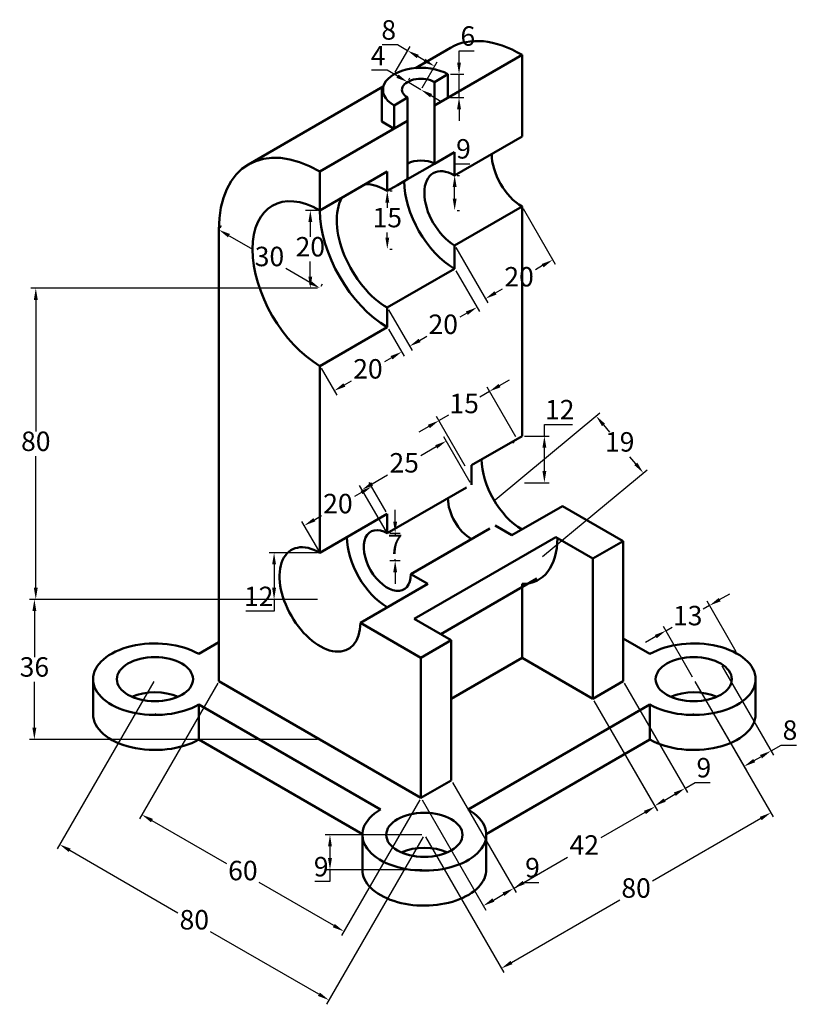
# Model space of a CAD drawing. Units: millimetres. Extents: x 11 to 211, y -6 to 247.
import ezdxf

# ---------------------------------------------------------------- set-up
doc = ezdxf.new("R2010")
doc.units = ezdxf.units.MM
doc.layers.add('M-DIMS', color=2, linetype='Continuous', lineweight=25)
doc.layers.add('M-OUTL', color=7, linetype='Continuous', lineweight=50)
doc.styles.get("Standard").update_dxf_attribs({"font": 'arial.ttf'})
doc.dimstyles.new('ISO-25', dxfattribs={"dimtxt": 5, "dimasz": 3, "dimexe": 1.25, "dimexo": 0.625, "dimtad": 1, "dimtih": 1, "dimtoh": 1, "dimtxsty": 'Standard', "dimcen": 2.5, "dimadec": 0, "dimazin": 0, "dimtfac": 1, "dimtmove": 0, "dimatfit": 3, "dimfxl": 1, "dimarcsym": 0})

# ---------------------------------------------------------------- blocks, each defined once
blk = doc.blocks.new('*D1')
at = {"layer": 'Defpoints', "color": 0, "transparency": 16777216}
for p in [(183.96, 77.16), (203.77, 42.84), (114.67, 37.16)]:
    blk.add_point(p, dxfattribs=at)
at = {"layer": 'M-DIMS', "color": 0, "lineweight": -2, "transparency": 16777216}
for p, q in [((184.27, 76.61), (204.39, 41.76)), ((201.17, 41.34), (173.33, 25.27)), ((114.99, 36.61), (135.11, 1.76)), ((137.08, 4.34), (164.93, 20.41))]:
    blk.add_line(p, q, dxfattribs=at)
at = {"layer": 'M-DIMS', "color": 0, "transparency": 16777216}
for points in [[(200.92, 41.77), (201.42, 40.91), (203.77, 42.84)], [(136.83, 4.77), (137.33, 3.91), (134.49, 2.84)]]:
    blk.add_solid(points, dxfattribs=at)
at = {"layer": 'M-DIMS', "color": 0, "transparency": 16777216, "insert": (169.13, 22.84), "char_height": 5, "attachment_point": 5}
blk.add_mtext('80', dxfattribs=at)
blk = doc.blocks.new('*D2')
at = {"layer": 'Defpoints', "color": 0, "transparency": 16777216}
for p in [(157.98, 72.16), (121.6, 51.16), (174, 44.4)]:
    blk.add_point(p, dxfattribs=at)
at = {"layer": 'M-DIMS', "color": 0, "lineweight": -2, "transparency": 16777216}
for p, q in [((158.29, 71.61), (174.62, 43.32)), ((121.91, 50.61), (138.25, 22.32)), ((171.4, 42.9), (160.09, 36.37)), ((140.22, 24.9), (151.53, 31.43))]:
    blk.add_line(p, q, dxfattribs=at)
at = {"layer": 'M-DIMS', "color": 0, "transparency": 16777216}
for points in [[(171.15, 43.33), (171.65, 42.47), (174, 44.4)], [(139.97, 25.33), (140.47, 24.47), (137.63, 23.4)]]:
    blk.add_solid(points, dxfattribs=at)
at = {"layer": 'M-DIMS', "color": 0, "transparency": 16777216, "insert": (155.81, 33.9), "char_height": 5, "attachment_point": 5}
blk.add_mtext('42', dxfattribs=at)
blk = doc.blocks.new('*D3')
at = {"layer": 'Defpoints', "color": 0, "transparency": 16777216}
for p in [(121.6, 51.16), (113.81, 46.66), (137.63, 23.4)]:
    blk.add_point(p, dxfattribs=at)
at = {"layer": 'M-DIMS', "color": 0, "lineweight": -2, "transparency": 16777216}
for p, q in [((121.91, 50.61), (138.25, 22.32)), ((114.12, 46.11), (130.46, 17.82)), ((137.63, 23.4), (140.22, 24.9)), ((140.22, 24.9), (144.14, 24.9)), ((132.43, 20.4), (135.03, 21.9))]:
    blk.add_line(p, q, dxfattribs=at)
at = {"layer": 'M-DIMS', "color": 0, "transparency": 16777216}
for points in [[(134.78, 22.33), (135.28, 21.47), (137.63, 23.4)], [(132.18, 20.83), (132.68, 19.97), (129.83, 18.9)]]:
    blk.add_solid(points, dxfattribs=at)
at = {"layer": 'M-DIMS', "color": 0, "transparency": 16777216, "insert": (142.49, 28.08), "char_height": 5, "attachment_point": 5}
blk.add_mtext('9', dxfattribs=at)
blk = doc.blocks.new('*D4')
at = {"layer": 'Defpoints', "color": 0, "transparency": 16777216}
for p in [(165.77, 76.66), (157.98, 72.16), (181.68, 49.09)]:
    blk.add_point(p, dxfattribs=at)
at = {"layer": 'M-DIMS', "color": 0, "lineweight": -2, "transparency": 16777216}
for p, q in [((166.08, 76.11), (182.31, 48.01)), ((158.29, 71.61), (174.51, 43.51)), ((181.68, 49.09), (184.28, 50.59)), ((184.28, 50.59), (188.19, 50.59)), ((176.49, 46.09), (179.08, 47.59))]:
    blk.add_line(p, q, dxfattribs=at)
at = {"layer": 'M-DIMS', "color": 0, "transparency": 16777216}
for points in [[(178.83, 48.03), (179.33, 47.16), (181.68, 49.09)], [(176.24, 46.53), (176.74, 45.66), (173.89, 44.59)]]:
    blk.add_solid(points, dxfattribs=at)
at = {"layer": 'M-DIMS', "color": 0, "transparency": 16777216, "insert": (186.55, 53.77), "char_height": 5, "attachment_point": 5}
blk.add_mtext('9', dxfattribs=at)
blk = doc.blocks.new('*D5')
at = {"layer": 'Defpoints', "color": 0, "transparency": 16777216}
for p in [(114.67, 37.16), (90.41, 28.16), (114.67, 28.16)]:
    blk.add_point(p, dxfattribs=at)
at = {"layer": 'M-DIMS', "color": 0, "lineweight": -2, "transparency": 16777216}
for p, q in [((114.05, 37.16), (89.16, 37.16)), ((90.41, 34.16), (90.41, 31.16)), ((114.05, 28.16), (89.16, 28.16)), ((90.41, 28.16), (90.41, 25.16)), ((90.41, 25.16), (86.49, 25.16))]:
    blk.add_line(p, q, dxfattribs=at)
at = {"layer": 'M-DIMS', "color": 0, "transparency": 16777216}
for points in [[(89.91, 34.16), (90.91, 34.16), (90.41, 37.16)], [(89.91, 31.16), (90.91, 31.16), (90.41, 28.16)]]:
    blk.add_solid(points, dxfattribs=at)
at = {"layer": 'M-DIMS', "color": 0, "transparency": 16777216, "insert": (88.14, 28.33), "char_height": 5, "attachment_point": 5}
blk.add_mtext('9', dxfattribs=at)
blk = doc.blocks.new('*D6')
at = {"layer": 'Defpoints', "color": 0, "transparency": 16777216}
for p in [(45.39, 77.16), (114.67, 37.16), (90.15, -5.32)]:
    blk.add_point(p, dxfattribs=at)
at = {"layer": 'M-DIMS', "color": 0, "lineweight": -2, "transparency": 16777216}
for p, q in [((45.08, 76.61), (20.24, 33.6)), ((114.36, 36.61), (89.53, -6.4)), ((23.47, 33.18), (51.31, 17.1)), ((87.55, -3.82), (59.71, 12.25))]:
    blk.add_line(p, q, dxfattribs=at)
at = {"layer": 'M-DIMS', "color": 0, "transparency": 16777216}
for points in [[(23.72, 33.61), (23.22, 32.75), (20.87, 34.68)], [(87.8, -3.39), (87.3, -4.25), (90.15, -5.32)]]:
    blk.add_solid(points, dxfattribs=at)
at = {"layer": 'M-DIMS', "color": 0, "transparency": 16777216, "insert": (55.51, 14.68), "char_height": 5, "attachment_point": 5}
blk.add_mtext('80', dxfattribs=at)
blk = doc.blocks.new('*D7')
at = {"layer": 'Defpoints', "color": 0, "transparency": 16777216}
for p in [(61.85, 76.66), (113.81, 46.66), (93.99, 12.33)]:
    blk.add_point(p, dxfattribs=at)
at = {"layer": 'M-DIMS', "color": 0, "lineweight": -2, "transparency": 16777216}
for p, q in [((61.53, 76.11), (41.4, 41.24)), ((113.5, 46.11), (93.36, 11.24)), ((44.62, 40.83), (63.8, 29.76)), ((91.39, 13.83), (72.22, 24.89))]:
    blk.add_line(p, q, dxfattribs=at)
at = {"layer": 'M-DIMS', "color": 0, "transparency": 16777216}
for points in [[(44.87, 41.26), (44.37, 40.39), (42.03, 42.33)], [(91.64, 14.26), (91.14, 13.39), (93.99, 12.33)]]:
    blk.add_solid(points, dxfattribs=at)
at = {"layer": 'M-DIMS', "color": 0, "transparency": 16777216, "insert": (68.01, 27.33), "char_height": 5, "attachment_point": 5}
blk.add_mtext('60', dxfattribs=at)
blk = doc.blocks.new('*D8')
at = {"layer": 'Defpoints', "color": 0, "transparency": 16777216}
for p in [(87.83, 177.66), (14.75, 97.66), (87.83, 97.66)]:
    blk.add_point(p, dxfattribs=at)
at = {"layer": 'M-DIMS', "color": 0, "lineweight": -2, "transparency": 16777216}
for p, q in [((87.2, 177.66), (13.5, 177.66)), ((14.75, 174.66), (14.75, 140.83)), ((14.75, 100.66), (14.75, 134.48)), ((87.2, 97.66), (13.5, 97.66))]:
    blk.add_line(p, q, dxfattribs=at)
at = {"layer": 'M-DIMS', "color": 0, "transparency": 16777216}
for points in [[(14.25, 174.66), (15.25, 174.66), (14.75, 177.66)], [(14.25, 100.66), (15.25, 100.66), (14.75, 97.66)]]:
    blk.add_solid(points, dxfattribs=at)
at = {"layer": 'M-DIMS', "color": 0, "transparency": 16777216, "insert": (14.75, 137.66), "char_height": 5, "attachment_point": 5}
blk.add_mtext('80', dxfattribs=at)
blk = doc.blocks.new('*D9')
at = {"layer": 'Defpoints', "color": 0, "transparency": 16777216}
for p in [(87.83, 97.66), (14.39, 61.66), (87.83, 61.66)]:
    blk.add_point(p, dxfattribs=at)
at = {"layer": 'M-DIMS', "color": 0, "lineweight": -2, "transparency": 16777216}
for p, q in [((87.2, 97.66), (13.14, 97.66)), ((14.39, 94.66), (14.39, 82.84)), ((14.39, 64.66), (14.39, 76.48)), ((87.2, 61.66), (13.14, 61.66))]:
    blk.add_line(p, q, dxfattribs=at)
at = {"layer": 'M-DIMS', "color": 0, "transparency": 16777216}
for points in [[(13.89, 94.66), (14.89, 94.66), (14.39, 97.66)], [(13.89, 64.66), (14.89, 64.66), (14.39, 61.66)]]:
    blk.add_solid(points, dxfattribs=at)
at = {"layer": 'M-DIMS', "color": 0, "transparency": 16777216, "insert": (14.39, 79.66), "char_height": 5, "attachment_point": 5}
blk.add_mtext('36', dxfattribs=at)
blk = doc.blocks.new('*D10')
at = {"layer": 'Defpoints', "color": 0, "transparency": 16777216}
for p in [(87.83, 109.66), (76.03, 97.66), (87.83, 97.66)]:
    blk.add_point(p, dxfattribs=at)
at = {"layer": 'M-DIMS', "color": 0, "lineweight": -2, "transparency": 16777216}
for p, q in [((87.2, 109.66), (74.78, 109.66)), ((76.03, 106.66), (76.03, 100.66)), ((87.2, 97.66), (74.78, 97.66)), ((76.03, 97.66), (76.03, 94.66)), ((76.03, 94.66), (68.76, 94.66))]:
    blk.add_line(p, q, dxfattribs=at)
at = {"layer": 'M-DIMS', "color": 0, "transparency": 16777216}
for points in [[(75.53, 106.66), (76.53, 106.66), (76.03, 109.66)], [(75.53, 100.66), (76.53, 100.66), (76.03, 97.66)]]:
    blk.add_solid(points, dxfattribs=at)
at = {"layer": 'M-DIMS', "color": 0, "transparency": 16777216, "insert": (72.08, 97.79), "char_height": 5, "attachment_point": 5}
blk.add_mtext('12', dxfattribs=at)
blk = doc.blocks.new('*D11')
at = {"layer": 'Defpoints', "color": 0, "transparency": 16777216}
for p in [(105.15, 114.66), (107.17, 114.66), (105.15, 107.66)]:
    blk.add_point(p, dxfattribs=at)
at = {"layer": 'M-DIMS', "color": 0, "lineweight": -2, "transparency": 16777216}
for p, q in [((107.17, 117.66), (107.17, 120.66)), ((105.77, 114.66), (108.42, 114.66)), ((107.17, 114.66), (107.17, 114.28)), ((105.77, 107.66), (108.42, 107.66)), ((107.17, 107.66), (107.17, 108.03)), ((107.17, 104.66), (107.17, 101.66))]:
    blk.add_line(p, q, dxfattribs=at)
at = {"layer": 'M-DIMS', "color": 0, "transparency": 16777216}
for points in [[(106.67, 117.66), (107.67, 117.66), (107.17, 114.66)], [(106.67, 104.66), (107.67, 104.66), (107.17, 107.66)]]:
    blk.add_solid(points, dxfattribs=at)
at = {"layer": 'M-DIMS', "color": 0, "transparency": 16777216, "insert": (107.17, 111.16), "char_height": 5, "attachment_point": 5}
blk.add_mtext('7', dxfattribs=at)
blk = doc.blocks.new('*D12')
at = {"layer": 'Defpoints', "color": 0, "transparency": 16777216}
for p in [(101.11, 126.65), (105.15, 119.66), (87.83, 109.66)]:
    blk.add_point(p, dxfattribs=at)
at = {"layer": 'M-DIMS', "color": 0, "lineweight": -2, "transparency": 16777216}
for p, q in [((104.84, 120.2), (100.49, 127.73)), ((98.51, 125.15), (96.69, 124.1)), ((86.39, 118.15), (88.21, 119.2)), ((87.51, 110.2), (83.16, 117.73))]:
    blk.add_line(p, q, dxfattribs=at)
at = {"layer": 'M-DIMS', "color": 0, "transparency": 16777216}
for points in [[(98.26, 125.58), (98.76, 124.72), (101.11, 126.65)], [(86.14, 118.58), (86.64, 117.72), (83.79, 116.65)]]:
    blk.add_solid(points, dxfattribs=at)
at = {"layer": 'M-DIMS', "color": 0, "transparency": 16777216, "insert": (92.45, 121.65), "char_height": 5, "attachment_point": 5}
blk.add_mtext('20', dxfattribs=at)
blk = doc.blocks.new('*D13')
at = {"layer": 'Defpoints', "color": 0, "transparency": 16777216}
for p in [(120.32, 138.38), (126.8, 127.16), (105.15, 114.66)]:
    blk.add_point(p, dxfattribs=at)
at = {"layer": 'M-DIMS', "color": 0, "lineweight": -2, "transparency": 16777216}
for p, q in [((126.49, 127.7), (119.69, 139.46)), ((117.72, 136.88), (113.76, 134.59)), ((101.27, 127.38), (105.23, 129.67)), ((104.84, 115.2), (98.04, 126.96))]:
    blk.add_line(p, q, dxfattribs=at)
at = {"layer": 'M-DIMS', "color": 0, "transparency": 16777216}
for points in [[(117.47, 137.31), (117.97, 136.45), (120.32, 138.38)], [(101.02, 127.81), (101.52, 126.95), (98.67, 125.88)]]:
    blk.add_solid(points, dxfattribs=at)
at = {"layer": 'M-DIMS', "color": 0, "transparency": 16777216, "insert": (109.49, 132.13), "char_height": 5, "attachment_point": 5}
blk.add_mtext('25', dxfattribs=at)
blk = doc.blocks.new('*D14')
at = {"layer": 'Defpoints', "color": 0, "transparency": 16777216}
for p in [(131.42, 151.13), (138.48, 138.9), (125.49, 131.4)]:
    blk.add_point(p, dxfattribs=at)
at = {"layer": 'M-DIMS', "color": 0, "lineweight": -2, "transparency": 16777216}
for p, q in [((138.16, 139.44), (130.79, 152.21)), ((134.02, 152.63), (136.61, 154.13)), ((131.42, 151.13), (128.91, 149.68)), ((125.17, 131.94), (117.8, 144.71)), ((118.43, 143.63), (120.93, 145.07)), ((115.83, 142.13), (113.23, 140.63))]:
    blk.add_line(p, q, dxfattribs=at)
at = {"layer": 'M-DIMS', "color": 0, "transparency": 16777216}
for points in [[(133.77, 153.06), (134.27, 152.19), (131.42, 151.13)], [(115.58, 142.56), (116.08, 141.69), (118.43, 143.63)]]:
    blk.add_solid(points, dxfattribs=at)
at = {"layer": 'M-DIMS', "color": 0, "transparency": 16777216, "insert": (124.92, 147.38), "char_height": 5, "attachment_point": 5}
blk.add_mtext('15', dxfattribs=at)
blk = doc.blocks.new('*D15')
at = {"layer": 'Defpoints', "color": 0, "transparency": 16777216}
for p in [(139.79, 139.66), (145.55, 139.66), (139.79, 127.66)]:
    blk.add_point(p, dxfattribs=at)
at = {"layer": 'M-DIMS', "color": 0, "lineweight": -2, "transparency": 16777216}
for p, q in [((145.55, 139.66), (145.55, 142.66)), ((145.55, 142.66), (152.81, 142.66)), ((140.41, 139.66), (146.8, 139.66)), ((145.55, 130.66), (145.55, 136.66)), ((140.41, 127.66), (146.8, 127.66))]:
    blk.add_line(p, q, dxfattribs=at)
at = {"layer": 'M-DIMS', "color": 0, "transparency": 16777216}
for points in [[(145.05, 136.66), (146.05, 136.66), (145.55, 139.66)], [(145.05, 130.66), (146.05, 130.66), (145.55, 127.66)]]:
    blk.add_solid(points, dxfattribs=at)
at = {"layer": 'M-DIMS', "color": 0, "transparency": 16777216, "insert": (149.49, 145.79), "char_height": 5, "attachment_point": 5}
blk.add_mtext('12', dxfattribs=at)
blk = doc.blocks.new('*D16')
at = {"layer": 'Defpoints', "color": 0, "transparency": 16777216}
for p in [(105.15, 167.66), (108.83, 161.28), (87.83, 157.66)]:
    blk.add_point(p, dxfattribs=at)
at = {"layer": 'M-DIMS', "color": 0, "lineweight": -2, "transparency": 16777216}
for p, q in [((105.46, 167.11), (109.45, 160.2)), ((106.23, 159.78), (104.41, 158.73)), ((88.14, 157.11), (92.13, 150.2)), ((94.1, 152.78), (95.93, 153.84))]:
    blk.add_line(p, q, dxfattribs=at)
at = {"layer": 'M-DIMS', "color": 0, "transparency": 16777216}
for points in [[(105.98, 160.22), (106.48, 159.35), (108.83, 161.28)], [(93.85, 153.22), (94.35, 152.35), (91.51, 151.28)]]:
    blk.add_solid(points, dxfattribs=at)
at = {"layer": 'M-DIMS', "color": 0, "transparency": 16777216, "insert": (100.17, 156.28), "char_height": 5, "attachment_point": 5}
blk.add_mtext('20', dxfattribs=at)
blk = doc.blocks.new('*D17')
at = {"layer": 'Defpoints', "color": 0, "transparency": 16777216}
for p in [(122.47, 182.66), (105.15, 172.66), (128.2, 172.74)]:
    blk.add_point(p, dxfattribs=at)
at = {"layer": 'M-DIMS', "color": 0, "lineweight": -2, "transparency": 16777216}
for p, q in [((122.78, 182.11), (128.82, 171.65)), ((105.46, 172.11), (111.5, 161.65)), ((125.6, 171.24), (123.78, 170.18)), ((113.47, 164.24), (115.29, 165.29))]:
    blk.add_line(p, q, dxfattribs=at)
at = {"layer": 'M-DIMS', "color": 0, "transparency": 16777216}
for points in [[(125.35, 171.67), (125.85, 170.8), (128.2, 172.74)], [(113.22, 164.67), (113.72, 163.8), (110.87, 162.74)]]:
    blk.add_solid(points, dxfattribs=at)
at = {"layer": 'M-DIMS', "color": 0, "transparency": 16777216, "insert": (119.53, 167.74), "char_height": 5, "attachment_point": 5}
blk.add_mtext('20', dxfattribs=at)
blk = doc.blocks.new('*D18')
at = {"layer": 'Defpoints', "color": 0, "transparency": 16777216}
for p in [(139.79, 198.66), (122.47, 188.66), (147.7, 184.95)]:
    blk.add_point(p, dxfattribs=at)
at = {"layer": 'M-DIMS', "color": 0, "lineweight": -2, "transparency": 16777216}
for p, q in [((140.1, 198.11), (148.33, 183.87)), ((122.78, 188.11), (131.01, 173.87)), ((145.1, 183.45), (143.28, 182.4)), ((132.98, 176.45), (134.8, 177.5))]:
    blk.add_line(p, q, dxfattribs=at)
at = {"layer": 'M-DIMS', "color": 0, "transparency": 16777216}
for points in [[(144.85, 183.88), (145.35, 183.02), (147.7, 184.95)], [(132.73, 176.88), (133.23, 176.02), (130.38, 174.95)]]:
    blk.add_solid(points, dxfattribs=at)
at = {"layer": 'M-DIMS', "color": 0, "transparency": 16777216, "insert": (139.04, 179.95), "char_height": 5, "attachment_point": 5}
blk.add_mtext('20', dxfattribs=at)
blk = doc.blocks.new('*D19')
at = {"layer": 'Defpoints', "color": 0, "transparency": 16777216}
for p in [(170.97, 130.2), (132.43, 122.9), (144.57, 108.28)]:
    blk.add_point(p, dxfattribs=at)
at = {"layer": 'M-DIMS', "color": 0, "lineweight": -2, "transparency": 16777216}
for p, q in [((132.92, 123.3), (159.8, 145.62)), ((160.76, 142.51), (162.27, 140.69)), ((169.06, 132.51), (167.54, 134.33)), ((145.05, 108.68), (171.94, 131))]:
    blk.add_line(p, q, dxfattribs=at)
at = {"layer": 'M-DIMS', "color": 0, "transparency": 16777216}
for points in [[(161.14, 142.83), (160.37, 142.19), (158.84, 144.82)], [(169.44, 132.83), (168.67, 132.19), (170.97, 130.2)]]:
    blk.add_solid(points, dxfattribs=at)
at = {"layer": 'M-DIMS', "color": 0, "transparency": 16777216, "insert": (164.91, 137.51), "char_height": 5, "attachment_point": 5}
blk.add_mtext('19', dxfattribs=at)
blk = doc.blocks.new('*D20')
at = {"layer": 'Defpoints', "color": 0, "transparency": 16777216}
for p in [(61.85, 192.66), (61.85, 192.66), (87.83, 177.66)]:
    blk.add_point(p, dxfattribs=at)
at = {"layer": 'M-DIMS', "color": 0, "lineweight": -2, "transparency": 16777216}
for p, q in [((62.16, 193.2), (62.47, 193.74)), ((64.44, 191.16), (70.64, 187.58)), ((85.23, 179.16), (79.03, 182.73)), ((88.14, 178.2), (88.45, 178.74))]:
    blk.add_line(p, q, dxfattribs=at)
at = {"layer": 'M-DIMS', "color": 0, "transparency": 16777216}
for points in [[(64.69, 191.59), (64.19, 190.72), (61.85, 192.66)], [(85.48, 179.59), (84.98, 178.72), (87.83, 177.66)]]:
    blk.add_solid(points, dxfattribs=at)
at = {"layer": 'M-DIMS', "color": 0, "transparency": 16777216, "insert": (74.84, 185.16), "char_height": 5, "attachment_point": 5}
blk.add_mtext('30', dxfattribs=at)
blk = doc.blocks.new('*D21')
at = {"layer": 'Defpoints', "color": 0, "transparency": 16777216}
for p in [(85.35, 197.66), (87.83, 197.66), (87.83, 177.66)]:
    blk.add_point(p, dxfattribs=at)
at = {"layer": 'M-DIMS', "color": 0, "lineweight": -2, "transparency": 16777216}
for p, q in [((87.2, 197.66), (84.1, 197.66)), ((85.35, 194.66), (85.35, 190.83)), ((85.35, 180.66), (85.35, 184.48)), ((87.2, 177.66), (84.1, 177.66))]:
    blk.add_line(p, q, dxfattribs=at)
at = {"layer": 'M-DIMS', "color": 0, "transparency": 16777216}
for points in [[(84.85, 194.66), (85.85, 194.66), (85.35, 197.66)], [(84.85, 180.66), (85.85, 180.66), (85.35, 177.66)]]:
    blk.add_solid(points, dxfattribs=at)
at = {"layer": 'M-DIMS', "color": 0, "transparency": 16777216, "insert": (85.35, 187.66), "char_height": 5, "attachment_point": 5}
blk.add_mtext('20', dxfattribs=at)
blk = doc.blocks.new('*D22')
at = {"layer": 'Defpoints', "color": 0, "transparency": 16777216}
for p in [(105.15, 202.66), (105.15, 202.66), (105.15, 187.66)]:
    blk.add_point(p, dxfattribs=at)
at = {"layer": 'M-DIMS', "color": 0, "lineweight": -2, "transparency": 16777216}
for p, q in [((105.77, 202.66), (106.4, 202.66)), ((105.15, 199.66), (105.15, 198.33)), ((105.15, 190.66), (105.15, 191.98)), ((105.77, 187.66), (106.4, 187.66))]:
    blk.add_line(p, q, dxfattribs=at)
at = {"layer": 'M-DIMS', "color": 0, "transparency": 16777216}
for points in [[(104.65, 199.66), (105.65, 199.66), (105.15, 202.66)], [(104.65, 190.66), (105.65, 190.66), (105.15, 187.66)]]:
    blk.add_solid(points, dxfattribs=at)
at = {"layer": 'M-DIMS', "color": 0, "transparency": 16777216, "insert": (105.15, 195.16), "char_height": 5, "attachment_point": 5}
blk.add_mtext('15', dxfattribs=at)
blk = doc.blocks.new('*D23')
at = {"layer": 'Defpoints', "color": 0, "transparency": 16777216}
for p in [(122.47, 206.66), (122.47, 206.66), (122.47, 197.66)]:
    blk.add_point(p, dxfattribs=at)
at = {"layer": 'M-DIMS', "color": 0, "lineweight": -2, "transparency": 16777216}
for p, q in [((122.47, 206.66), (122.47, 209.66)), ((122.47, 209.66), (126.38, 209.66)), ((123.09, 206.66), (123.72, 206.66)), ((122.47, 200.66), (122.47, 203.66)), ((123.09, 197.66), (123.72, 197.66))]:
    blk.add_line(p, q, dxfattribs=at)
at = {"layer": 'M-DIMS', "color": 0, "transparency": 16777216}
for points in [[(121.97, 203.66), (122.97, 203.66), (122.47, 206.66)], [(121.97, 200.66), (122.97, 200.66), (122.47, 197.66)]]:
    blk.add_solid(points, dxfattribs=at)
at = {"layer": 'M-DIMS', "color": 0, "transparency": 16777216, "insert": (124.74, 212.83), "char_height": 5, "attachment_point": 5}
blk.add_mtext('9', dxfattribs=at)
blk = doc.blocks.new('*D24')
at = {"layer": 'Defpoints', "color": 0, "transparency": 16777216}
for p in [(120.74, 232.66), (123.59, 232.66), (120.74, 226.66)]:
    blk.add_point(p, dxfattribs=at)
at = {"layer": 'M-DIMS', "color": 0, "lineweight": -2, "transparency": 16777216}
for p, q in [((123.59, 235.66), (123.59, 238.66)), ((123.59, 238.66), (127.51, 238.66)), ((121.36, 232.66), (124.84, 232.66)), ((123.59, 226.66), (123.59, 232.66)), ((121.36, 226.66), (124.84, 226.66)), ((123.59, 223.66), (123.59, 220.66))]:
    blk.add_line(p, q, dxfattribs=at)
at = {"layer": 'M-DIMS', "color": 0, "transparency": 16777216}
for points in [[(123.09, 235.66), (124.09, 235.66), (123.59, 232.66)], [(123.09, 223.66), (124.09, 223.66), (123.59, 226.66)]]:
    blk.add_solid(points, dxfattribs=at)
at = {"layer": 'M-DIMS', "color": 0, "transparency": 16777216, "insert": (125.86, 241.83), "char_height": 5, "attachment_point": 5}
blk.add_mtext('6', dxfattribs=at)
blk = doc.blocks.new('*D25')
at = {"layer": 'Defpoints', "color": 0, "transparency": 16777216}
for p in [(110.34, 230.66), (110.34, 230.66), (113.81, 228.66)]:
    blk.add_point(p, dxfattribs=at)
at = {"layer": 'M-DIMS', "color": 0, "lineweight": -2, "transparency": 16777216}
for p, q in [((105.15, 233.66), (101.06, 233.66)), ((107.75, 232.16), (105.15, 233.66)), ((113.81, 228.66), (110.34, 230.66)), ((110.66, 231.2), (110.97, 231.74)), ((114.12, 229.2), (114.43, 229.74)), ((116.41, 227.16), (119, 225.66))]:
    blk.add_line(p, q, dxfattribs=at)
at = {"layer": 'M-DIMS', "color": 0, "transparency": 16777216}
for points in [[(108, 232.59), (107.5, 231.72), (110.34, 230.66)], [(116.66, 227.59), (116.16, 226.72), (113.81, 228.66)]]:
    blk.add_solid(points, dxfattribs=at)
at = {"layer": 'M-DIMS', "color": 0, "transparency": 16777216, "insert": (102.79, 236.78), "char_height": 5, "attachment_point": 5}
blk.add_mtext('4', dxfattribs=at)
blk = doc.blocks.new('*D26')
at = {"layer": 'Defpoints', "color": 0, "transparency": 16777216}
for p in [(110.38, 238.71), (106.88, 232.66), (113.81, 228.66)]:
    blk.add_point(p, dxfattribs=at)
at = {"layer": 'M-DIMS', "color": 0, "lineweight": -2, "transparency": 16777216}
for p, q in [((107.78, 240.21), (103.86, 240.21)), ((107.19, 233.2), (111, 239.8)), ((110.38, 238.71), (107.78, 240.21)), ((114.71, 236.21), (112.98, 237.21)), ((114.12, 229.2), (117.93, 235.8))]:
    blk.add_line(p, q, dxfattribs=at)
at = {"layer": 'M-DIMS', "color": 0, "transparency": 16777216}
for points in [[(113.23, 237.65), (112.73, 236.78), (110.38, 238.71)], [(114.96, 236.65), (114.46, 235.78), (117.31, 234.71)]]:
    blk.add_solid(points, dxfattribs=at)
at = {"layer": 'M-DIMS', "color": 0, "transparency": 16777216, "insert": (105.51, 243.39), "char_height": 5, "attachment_point": 5}
blk.add_mtext('8', dxfattribs=at)
blk = doc.blocks.new('*D27')
at = {"layer": 'Defpoints', "color": 0, "transparency": 16777216}
for p in [(188.03, 96.11), (195.21, 83.66), (183.96, 77.16)]:
    blk.add_point(p, dxfattribs=at)
at = {"layer": 'M-DIMS', "color": 0, "lineweight": -2, "transparency": 16777216}
for p, q in [((190.62, 97.61), (193.22, 99.11)), ((194.9, 84.2), (187.4, 97.19)), ((188.03, 96.11), (186.37, 95.15)), ((183.64, 77.7), (176.14, 90.69)), ((176.77, 89.61), (178.43, 90.56)), ((174.17, 88.11), (171.57, 86.61))]:
    blk.add_line(p, q, dxfattribs=at)
at = {"layer": 'M-DIMS', "color": 0, "transparency": 16777216}
for points in [[(190.37, 98.04), (190.87, 97.17), (188.03, 96.11)], [(173.92, 88.54), (174.42, 87.67), (176.77, 89.61)]]:
    blk.add_solid(points, dxfattribs=at)
at = {"layer": 'M-DIMS', "color": 0, "transparency": 16777216, "insert": (182.4, 92.86), "char_height": 5, "attachment_point": 5}
blk.add_mtext('13', dxfattribs=at)
blk = doc.blocks.new('*D28')
at = {"layer": 'Defpoints', "color": 0, "transparency": 16777216}
for p in [(190.88, 81.16), (183.96, 77.16), (203.83, 58.74)]:
    blk.add_point(p, dxfattribs=at)
at = {"layer": 'M-DIMS', "color": 0, "lineweight": -2, "transparency": 16777216}
for p, q in [((191.2, 80.61), (204.45, 57.65)), ((184.27, 76.61), (197.52, 53.65)), ((203.83, 58.74), (206.43, 60.24)), ((206.43, 60.24), (210.35, 60.24)), ((199.5, 56.24), (201.23, 57.24))]:
    blk.add_line(p, q, dxfattribs=at)
at = {"layer": 'M-DIMS', "color": 0, "transparency": 16777216}
for points in [[(200.98, 57.67), (201.48, 56.8), (203.83, 58.74)], [(199.25, 56.67), (199.75, 55.8), (196.9, 54.74)]]:
    blk.add_solid(points, dxfattribs=at)
at = {"layer": 'M-DIMS', "color": 0, "transparency": 16777216, "insert": (208.7, 63.42), "char_height": 5, "attachment_point": 5}
blk.add_mtext('8', dxfattribs=at)

msp = doc.modelspace()

# ---------------------------------------------------------------- linework, layer by layer
at = {"layer": 'M-OUTL'}
for p, q in [((112.369, 234.251), (121.418, 239.475)), ((117.272, 224.655), (139.789, 237.655)), ((139.789, 216.655), (139.789, 237.655)), ((117.272, 230.655), (120.736, 232.655)), ((117.272, 230.655), (117.272, 209.655)), ((120.736, 232.655), (120.736, 226.655)), ((69.456, 209.475), (104.116, 229.486)), ((103.733, 220.473), (103.733, 229.265)), ((104.116, 229.486), (104.116, 227.825)), ((110.344, 226.655), (106.88, 224.655)), ((110.344, 226.655), (110.344, 205.655)), ((106.88, 224.655), (106.88, 218.655)), ((87.827, 207.655), (110.344, 220.655)), ((106.88, 218.655), (103.733, 220.473)), ((106.88, 218.655), (106.88, 218.655)), ((122.468, 206.655), (139.789, 216.655)), ((117.272, 209.655), (122.468, 212.655)), ((122.468, 206.655), (122.468, 212.655)), ((87.827, 197.655), (87.827, 207.655)), ((87.827, 197.655), (105.148, 207.655)), ((105.148, 202.655), (105.148, 207.655)), ((110.344, 205.655), (117.272, 209.655)), ((110.344, 205.655), (107.762, 204.165)), ((105.148, 202.655), (107.762, 204.165)), ((122.468, 188.655), (139.789, 198.655)), ((139.789, 198.655), (139.789, 139.655)), ((61.847, 112.655), (61.847, 192.655)), ((122.468, 188.655), (122.468, 182.655)), ((105.148, 172.655), (122.468, 182.655)), ((105.148, 172.655), (105.148, 167.655)), ((87.827, 157.655), (105.148, 167.655)), ((87.827, 109.655), (87.827, 157.655)), ((126.799, 132.155), (139.789, 139.655)), ((126.798, 132.155), (126.798, 127.155)), ((105.148, 114.655), (125.487, 126.398)), ((137.191, 114.155), (150.181, 121.655)), ((165.77, 112.655), (150.181, 121.655)), ((87.827, 109.655), (105.148, 119.655)), ((105.148, 114.655), (105.148, 119.655)), ((137.191, 114.155), (132.86, 116.655)), ((111.21, 104.155), (131.549, 115.898)), ((61.847, 76.655), (61.847, 112.655)), ((112.076, 92.655), (148.449, 113.655)), ((157.975, 108.155), (148.449, 113.655)), ((165.77, 112.655), (157.975, 108.155)), ((165.77, 76.655), (165.77, 112.655)), ((157.975, 108.155), (157.975, 72.155)), ((111.21, 104.155), (115.54, 101.655)), ((98.22, 91.655), (115.54, 101.655)), ((143.629, 103.002), (118.891, 88.72)), ((139.789, 91.655), (139.789, 101.659)), ((139.789, 82.655), (139.789, 100.785)), ((113.808, 82.655), (98.22, 91.655)), ((121.602, 87.155), (112.076, 92.655)), ((56.65, 83.655), (61.847, 86.655)), ((113.808, 82.655), (121.602, 87.155)), ((121.602, 51.155), (121.602, 87.155)), ((172.698, 83.655), (165.77, 87.655)), ((113.808, 46.655), (113.808, 82.655)), ((121.602, 72.155), (139.789, 82.655)), ((157.975, 72.155), (139.789, 82.655)), ((29.47, 77.155), (29.47, 68.155)), ((113.808, 46.655), (61.847, 76.655)), ((157.975, 72.155), (165.77, 76.655)), ((199.878, 77.155), (199.878, 68.155)), ((103.416, 43.655), (56.65, 70.655)), ((56.65, 61.655), (56.65, 70.655)), ((125.933, 43.655), (172.698, 70.655)), ((172.698, 70.655), (172.698, 61.655)), ((45.392, 68.155), (45.722, 67.965)), ((183.626, 67.965), (183.956, 68.155)), ((183.956, 68.155), (183.956, 67.963)), ((56.65, 61.655), (98.756, 37.346)), ((130.592, 37.346), (172.698, 61.655)), ((113.808, 46.655), (121.602, 51.155)), ((113.808, 46.655), (113.808, 46.655)), ((98.753, 37.155), (98.753, 28.155)), ((130.592, 37.346), (130.592, 27.965))]:
    msp.add_line(p, q, dxfattribs=at)
for centre, major_axis, start_param, end_param in [((139.789, 207.655), (18.371, -31.82), 2.3561945, 3.1415927), ((113.808, 228.655), (-9.798, 0), 3.9269908, 7.0685835), ((113.808, 228.655), (-4.899, 0), 3.9269908, 7.0685835), ((87.827, 177.655), (18.371, -31.82), 2.3561945, 3.9269908), ((113.808, 207.655), (-4.899, 0), 3.9269908, 5.4977871), ((139.789, 207.655), (5.511, -9.546), 3.9269908, 5.4977871), ((122.468, 197.655), (5.511, -9.546), 2.3561945, 5.4977871), ((122.468, 197.655), (9.186, -15.91), 3.9269908, 5.4977871), ((87.827, 177.655), (12.247, -21.213), 2.3561945, 5.4977871), ((105.148, 187.655), (9.186, -15.91), 2.3561945, 2.8017557), ((105.148, 187.655), (9.186, -15.91), 3.4814296, 5.4977871), ((105.148, 187.655), (12.247, -21.213), 3.9269908, 5.4977871), ((132.434, 122.902), (11.635, -20.153), 2.0337511, 2.0549846), ((139.789, 127.655), (7.348, -12.728), 3.9269908, 5.4977871), ((126.798, 120.155), (4.287, -7.425), 3.9269908, 5.4977871), ((105.148, 107.655), (4.287, -7.425), 2.3561945, 7.0685835), ((87.827, 97.655), (7.348, -12.728), 2.3561945, 7.0685835), ((105.148, 107.655), (7.348, -12.728), 3.9269908, 5.4977871), ((132.434, 122.902), (11.635, -20.153), 5.9611521, 7.0685835), ((45.392, 77.155), (-15.922, 0), 3.9269908, 8.6393798), ((183.956, 77.155), (15.922, 0), 0, 2.3561945), ((183.956, 77.155), (15.922, 0), 3.9269908, 6.2831853), ((45.392, 68.155), (9.798, 0), 0.9198242, 2.2217684), ((183.956, 68.155), (9.798, 0), 0.9198242, 2.2217684), ((45.392, 68.155), (-15.922, 0), 6.2831853, 8.6393798), ((183.956, 68.155), (-15.922, 0), 7.0685835, 9.424778), ((114.674, 37.155), (-15.922, 0), 5.4977871, 10.2101761), ((114.674, 28.155), (-9.798, 0), 4.0614169, 5.3633611), ((114.674, 28.155), (-15.922, 0), 6.2831853, 9.4454939)]:
    msp.add_ellipse(centre, major_axis=major_axis, ratio=0.5773503, start_param=start_param, end_param=end_param, dxfattribs=at)
for centre in [(45.392, 77.155), (183.956, 77.155), (114.674, 37.155)]:
    msp.add_ellipse(centre, major_axis=(-9.798, 0), ratio=0.5773503, dxfattribs=at)

# ---------------------------------------------------------------- dimensions: what is measured, and where the dimension line sits
at = {"layer": 'M-DIMS'}
for p1, p2, distance, picture, middle in [((113.808, 228.655), (106.88, 232.655), -6.995, '*D26', (105.507, 243.391)), ((113.808, 228.655), (110.344, 230.655), 0, '*D25', (102.794, 236.78)), ((122.468, 188.655), (139.789, 198.655), -15.827, '*D18', (139.042, 179.949)), ((87.827, 177.655), (61.847, 192.655), 0, '*D20', (74.837, 185.155)), ((105.148, 172.655), (122.468, 182.655), -11.453, '*D17', (119.535, 167.736)), ((87.827, 157.655), (105.148, 167.655), -7.358, '*D16', (100.167, 156.283)), ((125.487, 131.398), (138.477, 138.898), 14.12, '*D14', (124.922, 147.376)), ((132.434, 122.902), (144.57, 108.282), 34.316, '*D19', (164.907, 137.51)), ((105.148, 114.655), (126.799, 127.155), 12.96, '*D13', (109.493, 132.129)), ((87.827, 109.655), (105.148, 119.655), 8.076, '*D12', (92.45, 121.649)), ((183.956, 77.155), (195.215, 83.655), 14.376, '*D27', (182.398, 92.855)), ((183.956, 77.155), (190.884, 81.155), -25.886, '*D28', (208.698, 63.415)), ((45.392, 77.155), (114.674, 37.155), -49.048, '*D6', (55.509, 14.678)), ((61.847, 76.655), (113.808, 46.655), -39.64, '*D7', (68.007, 27.326)), ((114.674, 37.155), (183.956, 77.155), -39.624, '*D1', (169.127, 22.84)), ((157.975, 72.155), (165.77, 76.655), -31.826, '*D4', (186.55, 53.771)), ((121.602, 51.155), (157.975, 72.155), -32.047, '*D2', (155.813, 33.902)), ((113.808, 46.655), (121.602, 51.155), -32.047, '*D3', (142.493, 28.079))]:
    dim = msp.add_aligned_dim(p1=p1, p2=p2, distance=distance, dimstyle='ISO-25', override={"dimclrd": 0, "dimclre": 0, "dimclrt": 0}, dxfattribs=at)
    dim.commit()
    dim.dimension.update_dxf_attribs({"geometry": picture, "text_midpoint": middle})
for base, p1, p2, picture, middle in [((123.587, 232.655), (120.736, 226.655), (120.736, 232.655), '*D24', (125.863, 241.833)), ((122.468, 206.655), (122.468, 197.655), (122.468, 206.655), '*D23', (124.737, 212.833)), ((105.148, 202.655), (105.148, 187.655), (105.148, 202.655), '*D22', (105.148, 195.155)), ((85.352, 197.655), (87.827, 177.655), (87.827, 197.655), '*D21', (85.352, 187.655)), ((14.746, 97.655), (87.827, 177.655), (87.827, 97.655), '*D8', (14.746, 137.655)), ((145.546, 139.655), (139.789, 127.655), (139.789, 139.655), '*D15', (149.491, 145.791)), ((107.174, 114.655), (105.148, 107.655), (105.148, 114.655), '*D11', (107.174, 111.155)), ((76.027, 97.655), (87.827, 109.655), (87.827, 97.655), '*D10', (72.082, 97.791)), ((14.395, 61.655), (87.827, 97.655), (87.827, 61.655), '*D9', (14.395, 79.655)), ((90.408, 28.155), (114.674, 37.155), (114.674, 28.155), '*D5', (88.139, 28.333))]:
    dim = msp.add_linear_dim(base=base, p1=p1, p2=p2, angle=90, dimstyle='ISO-25', override={"dimclrd": 0, "dimclre": 0, "dimclrt": 0}, dxfattribs=at)
    dim.commit()
    dim.dimension.update_dxf_attribs({"geometry": picture, "text_midpoint": middle})

doc.saveas('drawing.dxf')
